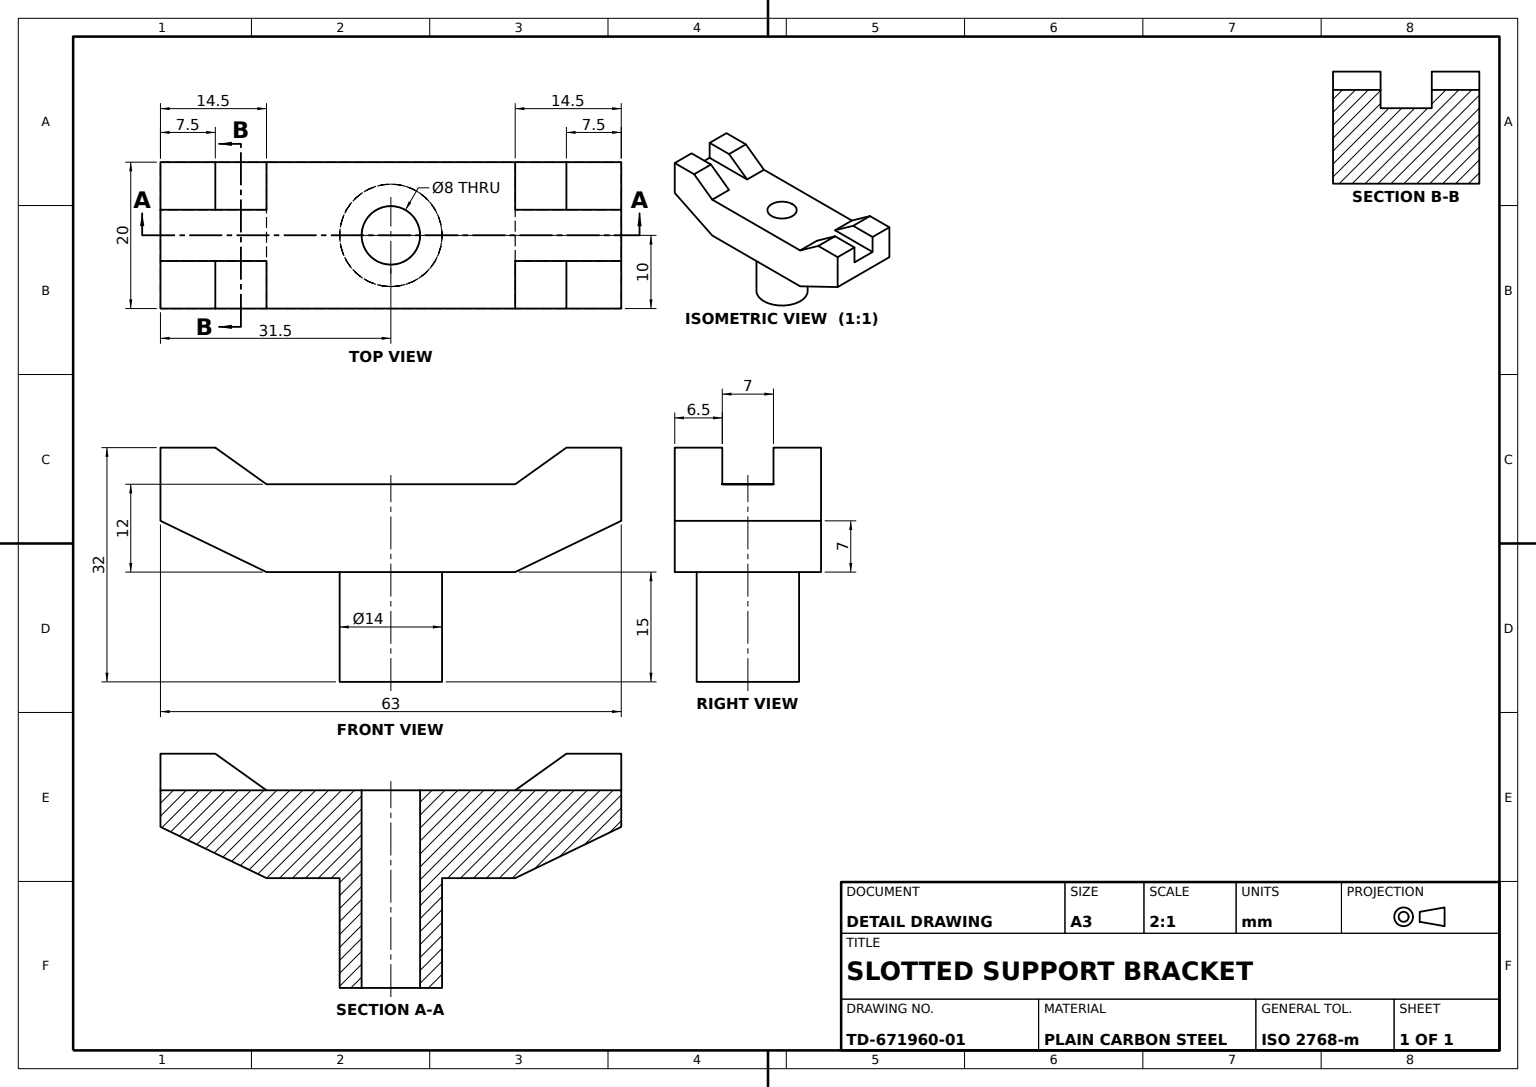
SolidWorks part; units mm, degrees
material "Plain Carbon Steel"
ref_plane "Front Plane" through (0, 0, 0) normal (0, 0, 1) x (1, 0, 0)
ref_plane "Top Plane" through (0, 0, 0) normal (0, 1, 0) x (1, 0, 0)
ref_plane "Right Plane" through (0, 0, 0) normal (1, 0, 0) x (0, 0, -1)
sketch "Base Profile Sketch" plane through (0, 0, 0) normal (0, 0, 1) x (1, 0, 0)
  line L0 (0, 0) -> (63, 0)
  line L2 (31.5, -12) -> (48.5, -12)
  line L3 (31.5, -12) -> (14.5, -12)
  line L4 (0, 0) -> (0, -5)
  line L5 (0, -5) -> (14.5, -12)
  line L6 (63, 0) -> (63, -5)
  line L7 (63, -5) -> (48.5, -12)
  dimension "D1" = 14.5
  dimension "D2" = 31.5
  dimension "D3" = 7
  dimension "D4" = 12
extrude "Base Block" add sketch "Base Profile Sketch" along normal blind 20
sketch "End Lugs Sketch" plane through (0, 0, 20) normal (0, 0, 1) x (1, 0, 0)
  line L0 (0, 0) -> (0, 5)
  line L1 (0, 5) -> (7.5, 5)
  line L2 (63, 0) -> (63, 5)
  line L3 (63, 5) -> (55.5, 5)
  line L4 (0, 0) -> (0, -5) construction
  line L5 (63, 0) -> (0, 0) construction
  line L6 (14.5, 0) -> (7.5, 5)
  line L7 (14.5, -12) -> (48.5, -12) construction
  line L8 (48.5, 0) -> (55.5, 5)
  line L9 (0, 0) -> (14.5, 0)
  line L10 (63, 0) -> (48.5, 0)
  dimension "D1" = 7.5
  dimension "D2" = 14.5
  dimension "D3" = 17
extrude "End Lugs" add sketch "End Lugs Sketch" against normal blind 20
sketch "Guide V-Slot Sketch" plane through (0, 0, 0) normal (-1, 0, 0) x (0, 0, 1)
  line L0 (10, 5) -> (6.5, 5)
  line L1 (0, 5) -> (20, 5) construction
  line L2 (6.5, 5) -> (6.5, 0)
  line L3 (6.5, 0) -> (13.5, 0)
  line L4 (13.5, 0) -> (13.5, 5)
  line L5 (13.5, 5) -> (10, 5)
  line L6 (0, 5) -> (0, -5) construction
  dimension "D1" = 6.5
extrude "Guide V-Slot" cut sketch "Guide V-Slot Sketch" against normal blind 63
sketch "Locating Pin Sketch Ø14" plane through (0, -12, 0) normal (0, -1, 0) x (1, 0, 0)
  line L0 (48.5, 20) -> (48.5, 0) construction
  line L1 (14.5, 0) -> (48.5, 0) construction
  circle A0 centre (31.5, 10) radius 7
  dimension "D1" = 14
  dimension "D2" = 14
  dimension "D3" = 17
  dimension "D4" = 10
extrude "Locating Pin Ø14" add sketch "Locating Pin Sketch Ø14" along normal blind 15
sketch "Hole Sketch Ø8" plane through (0, 0, 0) normal (0, 1, 0) x (1, 0, 0)
  line L0 (0, -6.5) -> (0, -13.5) construction
  line L1 (48.5, -20) -> (14.5, -20) construction
  circle A0 centre (31.5, -10) radius 4
  dimension "D1" = 8
  dimension "D2" = 8
  dimension "D3" = 31.5
  dimension "D4" = 10
extrude "Hole Ø8" cut sketch "Hole Sketch Ø8" against normal blind 32
